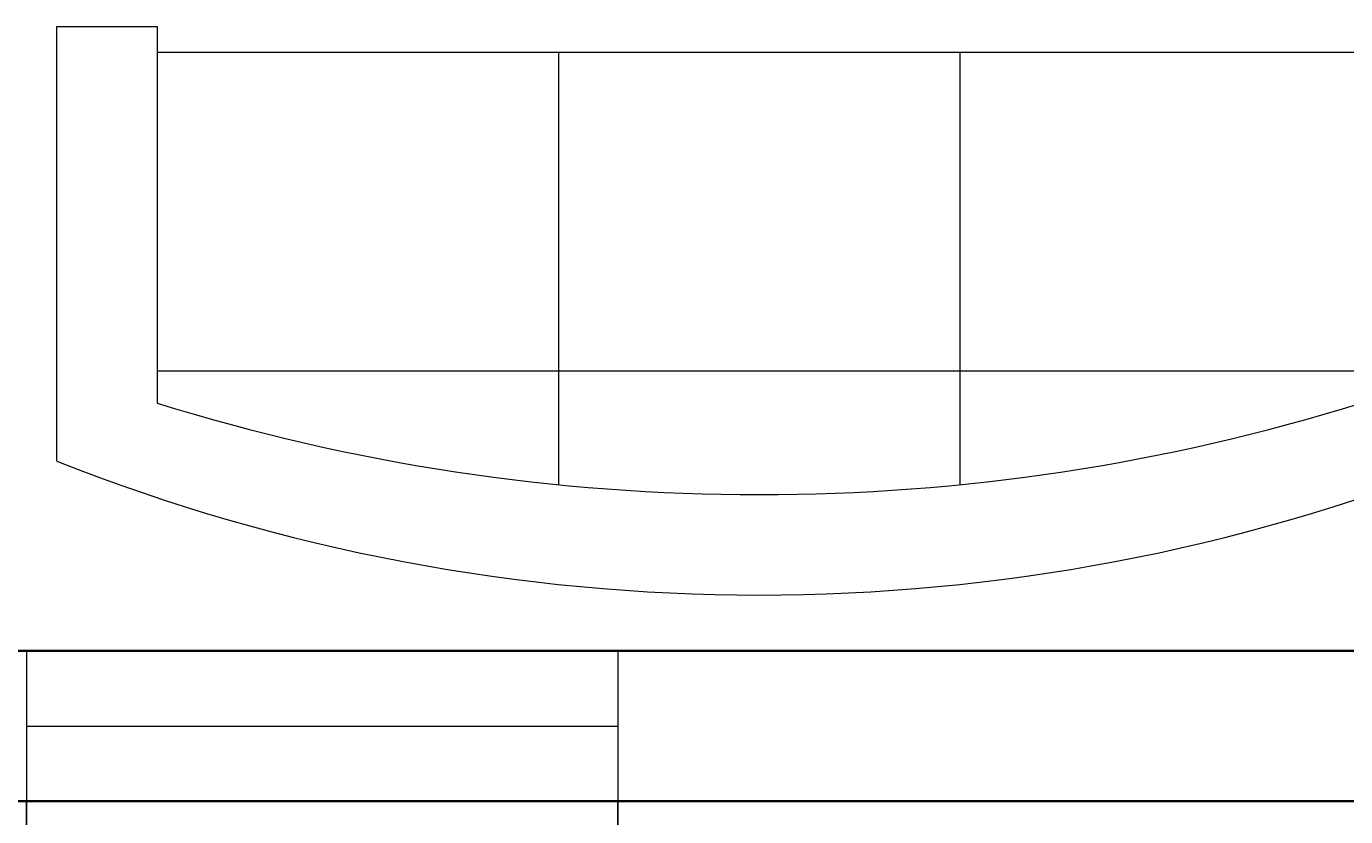
# Model space of a CAD drawing. Units: inches. Extents: x -86 to 2463, y -1058 to 68.
# Tile 10 of 17: x 69 to 148, y -304 to -257. Entities that reach past the tile are written whole.
import ezdxf

# ---------------------------------------------------------------- set-up
doc = ezdxf.new("R2010")
doc.units = ezdxf.units.IN
doc.header["$MEASUREMENT"] = 0
for name, color, linetype, lineweight in [('A-ANNO-DIMS', 2, 'Continuous', 18), ('A-FURN', 8, 'Continuous', 18), ('A-GLAZ', 4, 'Continuous', 18), ('A-WALL', 7, 'Continuous', 35)]:
    doc.layers.add(name, color=color, linetype=linetype, lineweight=lineweight)
doc.styles.get("Standard").update_dxf_attribs({"font": 'arial.ttf'})
doc.dimstyles.get("Standard").update_dxf_attribs({"dimtxt": 0.18, "dimasz": 0.18, "dimexe": 0.18, "dimexo": 0.0625, "dimgap": 0.09, "dimtad": 0, "dimtih": 1, "dimtoh": 1, "dimdec": 4, "dimzin": 0, "dimdsep": 46, "dimtxsty": 'Standard', "dimcen": 0.09, "dimadec": 0, "dimazin": 0, "dimtfac": 1, "dimtdec": 4, "dimtofl": 0, "dimtmove": 0, "dimatfit": 3, "dimfxl": 1, "dimtolj": 1, "dimtzin": 0, "dimarcsym": 0})

# ---------------------------------------------------------------- blocks, each defined once
blk = doc.blocks.new('Sofa - Roundback 7 ft.')
for p, q in [((-12.00002, -32.4421), (-12.00003, -6.5971)), ((11.99997, -32.4421), (11.99998, -6.5971)), ((-36.000027, -34), (-36.000027, -11.4696)), ((35.99998, -34), (35.99998, -11.4696)), ((-35.999844, -13.3819), (35.9998, -13.3819)), ((-36.000027, -32.4421), (35.99998, -32.4421))]:
    blk.add_line(p, q)
for points in [[(-36.000027, -34), (-42.000027, -34), (-42.000027, -8)], [(41.99998, -8), (41.99998, -34), (35.99998, -34)]]:
    blk.add_lwpolyline(points)
for centre, radius, start, end in [((0, -114.25), 114.25, 68.43141, 111.5686), ((-0.00001, -127.1968), 121.1968, 72.72033, 107.2797)]:
    blk.add_arc(centre, radius, start, end)
blk = doc.blocks.new('*D42')
at = {"layer": 'A-ANNO-DIMS', "color": 0, "lineweight": -2, "transparency": 16777216}
for p, q in [((68.889, -303.167), (68.889, -740.384)), ((104.261, -303.167), (104.261, -740.384)), ((69.069, -740.204), (86.181, -740.204)), ((104.081, -740.204), (86.969, -740.204))]:
    blk.add_line(p, q, dxfattribs=at)
at = {"layer": 'A-ANNO-DIMS', "color": 0, "transparency": 16777216}
for points in [[(69.069, -740.174), (69.069, -740.234), (68.889, -740.204)], [(104.081, -740.174), (104.081, -740.234), (104.261, -740.204)]]:
    blk.add_solid(points, dxfattribs=at)
at = {"layer": 'Defpoints', "color": 0, "transparency": 16777216}
for p in [(68.889, -303.104), (104.261, -303.104), (104.261, -740.204)]:
    blk.add_point(p, dxfattribs=at)
at = {"layer": 'A-ANNO-DIMS', "color": 0, "transparency": 16777216, "insert": (86.575, -740.204), "char_height": 0.18, "attachment_point": 5}
blk.add_mtext('\\A1;35.37', dxfattribs=at)

msp = doc.modelspace()

# ---------------------------------------------------------------- linework, layer by layer
at = {"layer": 'A-GLAZ'}
for p, q in [((68.889, -294.104), (68.889, -303.104)), ((104.261, -294.104), (104.261, -303.104)), ((68.889, -298.604), (104.261, -298.604))]:
    msp.add_line(p, q, dxfattribs=at)
at = {"layer": 'A-WALL'}
for p, q in [((183.761, -294.104), (24.761, -294.104)), ((377.846, -303.104), (15.761, -303.104))]:
    msp.add_line(p, q, dxfattribs=at)

# ---------------------------------------------------------------- block references
at = {"layer": 'A-FURN', "rotation": 180}
msp.add_blockref('Sofa - Roundback 7 ft.', (112.715, -290.771), dxfattribs=at)

# ---------------------------------------------------------------- dimensions: what is measured, and where the dimension line sits
at = {"layer": 'A-ANNO-DIMS'}
dim = msp.add_linear_dim(base=(104.261, -740.204), p1=(68.889, -303.104), p2=(104.261, -303.104), dimstyle='Standard', override={"dimdec": 2, "dimlfac": 1, "dimrnd": 0, "dimzin": 0, "dimdsep": 46, "dimlunit": 2}, dxfattribs=at)
dim.commit()
dim.dimension.update_dxf_attribs({"geometry": '*D42', "text_midpoint": (86.575, -740.204)})

doc.saveas('drawing.dxf')
